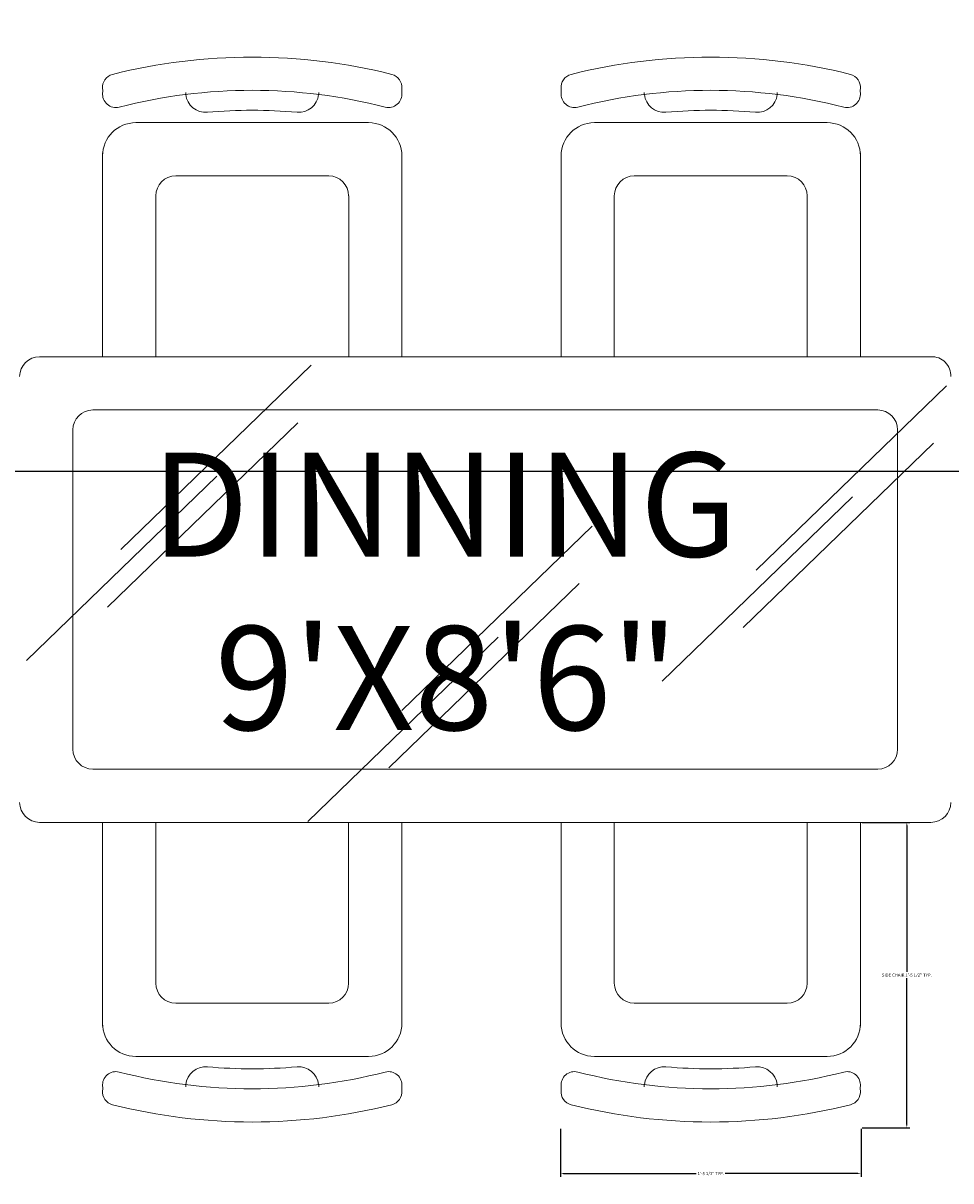
# Model space of a CAD drawing. Units: inches. Extents: x 182 to 1022, y -617 to 111.
# Tile 20 of 33: x 348 to 401, y -98 to -31. Entities that reach past the tile are written whole.
import ezdxf

# ---------------------------------------------------------------- set-up
doc = ezdxf.new("R2010")
doc.units = ezdxf.units.IN
doc.header["$MEASUREMENT"] = 0
doc.layers.add('A-ANNO-DIMS', color=2, linetype='Continuous', lineweight=18)
doc.layers.add('A-AREA-IDEN', color=8, linetype='Continuous', lineweight=18)
doc.layers.add('furniture', color=50, linetype='Continuous', lineweight=15, transparency=0.8)
doc.styles.get("Standard").update_dxf_attribs({"font": 'arial.ttf'})
doc.dimstyles.get("Standard").update_dxf_attribs({"dimtxt": 0.18, "dimasz": 0.18, "dimexe": 0.18, "dimexo": 0.0625, "dimgap": 0.09, "dimtad": 0, "dimtih": 1, "dimtoh": 1, "dimdec": 1, "dimzin": 0, "dimdsep": 46, "dimlunit": 4, "dimtxsty": 'Standard', "dimcen": 0.09, "dimadec": 0, "dimazin": 0, "dimtfac": 1, "dimtdec": 1, "dimtofl": 0, "dimtmove": 0, "dimatfit": 3, "dimfxl": 1, "dimtolj": 1, "dimtzin": 0, "dimarcsym": 0})

# ---------------------------------------------------------------- blocks, each defined once
blk = doc.blocks.new('DINING-CHAIR-SIDE')
for p, q in [((4.797, 15.128), (4.797, 15.25)), ((12.472, 15.128), (12.472, 15.25)), ((15.35, 13.501), (1.918, 13.501)), ((0, 11.757), (0, 11.361)), ((0, 11.582), (0, 0)), ((17.269, 11.361), (17.269, 11.757)), ((17.269, 0), (17.269, 11.582)), ((13.047, 10.431), (4.221, 10.431)), ((3.07, 9.279), (3.07, 0)), ((14.199, 0), (14.199, 9.279))]:
    blk.add_line(p, q)
for centre, radius, start, end in [((8.634, -15.67), 32.955, 75.85295, 104.14705), ((0.767, 15.541), 0.768, 104.14705, 185.92158), ((16.501, 15.541), 0.768, 354.07842, 75.85295), ((-1.141, 15.343), 1.151, 354.07842, 5.92158), ((8.634, -15.67), 31.036, 75.67863, 104.32137), ((18.41, 15.343), 1.151, 174.07842, 185.92158), ((0.767, 15.145), 0.768, 174.07842, 284.32137), ((5.948, 15.25), 1.151, 186.02809, 274.96535), ((11.32, 15.25), 1.151, 265.03465, 353.97191), ((16.501, 15.145), 0.768, 255.67863, 5.92158), ((8.634, -15.67), 29.885, 85.03465, 94.96535), ((1.918, 11.582), 1.919, 90, 180), ((15.35, 11.582), 1.919, 0, 90), ((4.221, 9.279), 1.151, 90, 180), ((13.047, 9.279), 1.151, 0, 90)]:
    blk.add_arc(centre, radius, start, end)
blk = doc.blocks.new('*D22')
at = {"layer": 'A-ANNO-DIMS', "color": 0, "lineweight": -2, "transparency": 16777216}
for p, q in [((396.072, -77.062), (398.832, -77.062)), ((398.652, -77.242), (398.652, -85.689)), ((398.652, -94.501), (398.652, -86.055)), ((396.072, -94.681), (398.832, -94.681))]:
    blk.add_line(p, q, dxfattribs=at)
at = {"layer": 'A-ANNO-DIMS', "color": 0, "transparency": 16777216}
for points in [[(398.622, -77.242), (398.682, -77.242), (398.652, -77.062)], [(398.622, -94.501), (398.682, -94.501), (398.652, -94.681)]]:
    blk.add_solid(points, dxfattribs=at)
at = {"layer": 'Defpoints', "color": 0, "transparency": 16777216}
for p in [(396.01, -77.062), (396.01, -94.681), (398.652, -94.681)]:
    blk.add_point(p, dxfattribs=at)
at = {"layer": 'A-ANNO-DIMS', "color": 0, "transparency": 16777216, "insert": (398.652, -85.872), "char_height": 0.18, "attachment_point": 5}
blk.add_mtext('\\A1;SIDE CHAIR 1\'-5 1/2" TYP.', dxfattribs=at)
blk = doc.blocks.new('*D23')
at = {"layer": 'A-ANNO-DIMS', "color": 0, "lineweight": -2, "transparency": 16777216}
for p, q in [((378.67, -94.743), (378.67, -97.504)), ((396.01, -94.743), (396.01, -97.504)), ((378.85, -97.324), (386.5, -97.324)), ((395.83, -97.324), (388.18, -97.324))]:
    blk.add_line(p, q, dxfattribs=at)
at = {"layer": 'A-ANNO-DIMS', "color": 0, "transparency": 16777216}
for points in [[(378.85, -97.294), (378.85, -97.354), (378.67, -97.324)], [(395.83, -97.294), (395.83, -97.354), (396.01, -97.324)]]:
    blk.add_solid(points, dxfattribs=at)
at = {"layer": 'Defpoints', "color": 0, "transparency": 16777216}
for p in [(378.67, -94.681), (396.01, -94.681), (378.67, -97.324)]:
    blk.add_point(p, dxfattribs=at)
at = {"layer": 'A-ANNO-DIMS', "color": 0, "transparency": 16777216, "insert": (387.34, -97.324), "char_height": 0.18, "attachment_point": 5}
blk.add_mtext('\\A1;1\'-5 1/2" TYP.', dxfattribs=at)
blk = doc.blocks.new('*D43')
at = {"layer": 'A-ANNO-DIMS', "color": 0, "lineweight": -2, "transparency": 16777216}
for p, q in [((556.299, -9.373), (186.381, -9.373)), ((186.561, -9.553), (186.561, -32.91)), ((186.561, -56.633), (186.561, -33.276)), ((556.299, -56.813), (186.381, -56.813))]:
    blk.add_line(p, q, dxfattribs=at)
at = {"layer": 'A-ANNO-DIMS', "color": 0, "transparency": 16777216}
for points in [[(186.531, -9.553), (186.591, -9.553), (186.561, -9.373)], [(186.531, -56.633), (186.591, -56.633), (186.561, -56.813)]]:
    blk.add_solid(points, dxfattribs=at)
at = {"layer": 'Defpoints', "color": 0, "transparency": 16777216}
for p in [(556.361, -9.373), (186.561, -56.813), (556.361, -56.813)]:
    blk.add_point(p, dxfattribs=at)
at = {"layer": 'A-ANNO-DIMS', "color": 0, "transparency": 16777216, "insert": (186.561, -33.093), "char_height": 0.18, "attachment_point": 5}
blk.add_mtext('\\A1;3\'-11 1/2"', dxfattribs=at)

msp = doc.modelspace()

# ---------------------------------------------------------------- linework, layer by layer
at = {"layer": 'furniture'}
for p, q in [((400.041, -50.199), (348.618, -50.199)), ((364.286, -50.697), (353.305, -61.329)), ((400.944, -51.879), (389.964, -62.511)), ((396.971, -53.269), (351.688, -53.269)), ((363.524, -54.01), (352.543, -64.642)), ((350.536, -54.421), (350.536, -72.841)), ((398.122, -72.841), (398.122, -54.421)), ((400.183, -55.191), (389.202, -65.823)), ((358.852, -57.1), (347.871, -67.732)), ((395.51, -58.281), (384.53, -68.913)), ((380.503, -59.979), (369.523, -70.611)), ((379.742, -63.292), (368.761, -73.924)), ((375.069, -66.381), (364.089, -77.013)), ((351.688, -73.992), (396.971, -73.992)), ((348.618, -77.062), (400.041, -77.062))]:
    msp.add_line(p, q, dxfattribs=at)
for centre, radius, start, end in [((348.618, -51.351), 1.151, 90, 180), ((400.095, -51.296), 1.098, 357.16604, 92.83396), ((351.688, -54.421), 1.151, 90, 180), ((396.971, -54.421), 1.151, 0, 90), ((351.688, -72.841), 1.151, 180, 270), ((396.971, -72.841), 1.151, 270, 0), ((348.618, -75.911), 1.151, 180, 270), ((400.041, -75.911), 1.151, 270, 0)]:
    msp.add_arc(centre, radius, start, end, dxfattribs=at)

# ---------------------------------------------------------------- block references
for p in [(352.251, -50.199), (378.706, -50.199)]:
    msp.add_blockref('DINING-CHAIR-SIDE', p, dxfattribs=at)
at = {"layer": 'furniture', "rotation": 180}
for p in [(369.519, -77.063), (395.974, -77.063)]:
    msp.add_blockref('DINING-CHAIR-SIDE', p, dxfattribs=at)

# ---------------------------------------------------------------- texts
at = {"layer": 'A-AREA-IDEN', "insert": (347.729, -55.734), "char_height": 6, "attachment_point": 1}
msp.add_mtext_dynamic_manual_height_columns('    DINNING\\P      9\'X8\'6"', width=53.39573, gutter_width=1, heights=[0], dxfattribs=at)

# ---------------------------------------------------------------- dimensions: what is measured, and where the dimension line sits
at = {"layer": 'A-ANNO-DIMS'}
dim = msp.add_linear_dim(base=(186.561, -56.813), p1=(556.361, -9.373), p2=(556.361, -56.813), angle=90, dimstyle='Standard', override={"dimdec": 1, "dimlfac": 1, "dimrnd": 0, "dimzin": 1, "dimdsep": 46, "dimlunit": 4, "dimfrac": 2}, dxfattribs=at)
dim.commit()
dim.dimension.update_dxf_attribs({"geometry": '*D43', "text_midpoint": (186.561, -33.093)})
for base, p1, p2, angle, text, picture, middle in [((398.652, -94.681), (396.01, -77.062), (396.01, -94.681), 270, 'SIDE CHAIR <> TYP.', '*D22', (398.652, -85.872)), ((378.67, -97.324), (396.01, -94.681), (378.67, -94.681), 180, '<> TYP.', '*D23', (387.34, -97.324))]:
    dim = msp.add_linear_dim(base=base, p1=p1, p2=p2, angle=angle, text=text, dimstyle='Standard', override={"dimdec": 1, "dimlfac": 1, "dimrnd": 0, "dimzin": 1, "dimdsep": 46, "dimlunit": 4, "dimfrac": 2}, dxfattribs=at)
    dim.commit()
    dim.dimension.update_dxf_attribs({"geometry": picture, "text_midpoint": middle})

doc.saveas('drawing.dxf')
